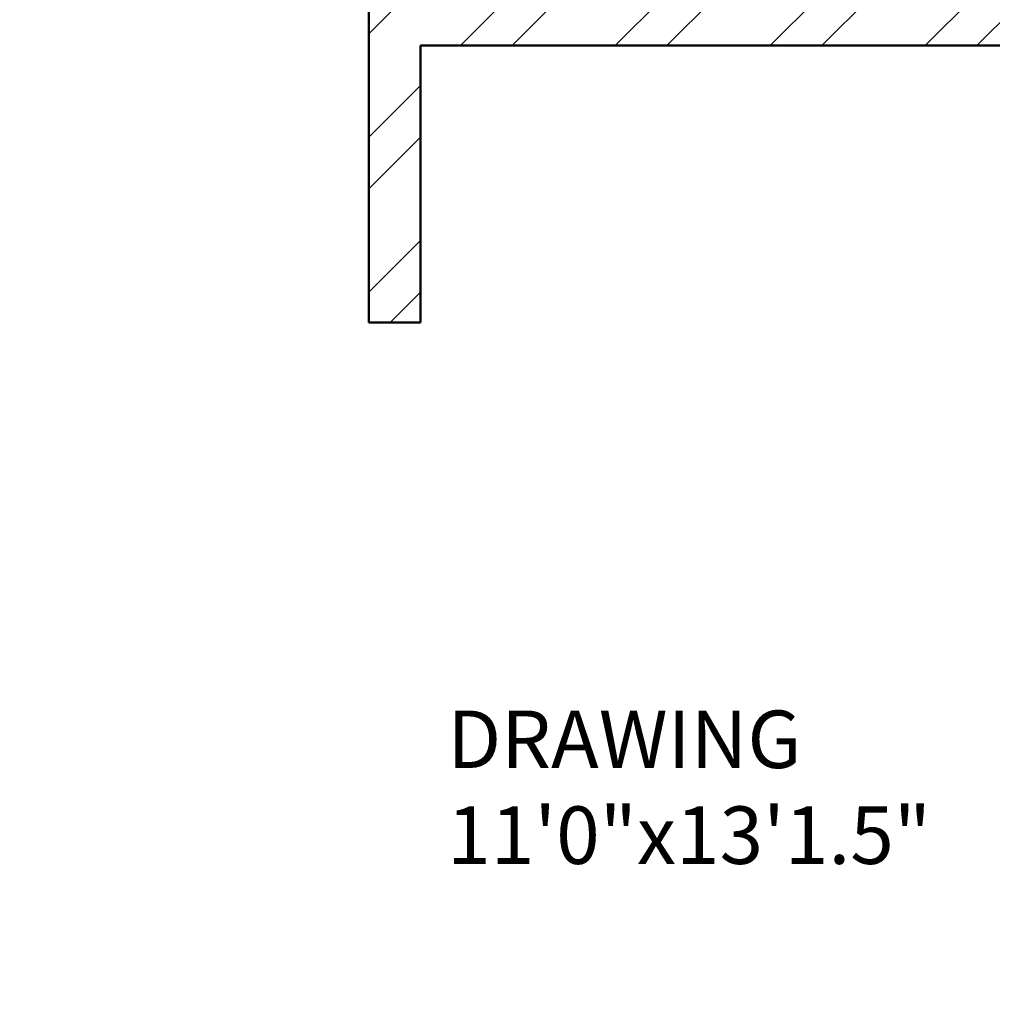
# Model space of a CAD drawing. Units: inches. Extents: x 963 to 2075, y 289 to 2657.
# Tile 73 of 98: x 1342 to 1426, y 2239 to 2325. Entities that reach past the tile are written whole.
import ezdxf

# ---------------------------------------------------------------- set-up
doc = ezdxf.new("R2010")
doc.units = ezdxf.units.IN
for name, color, linetype, lineweight in [('A-AREA-IDEN', 7, 'Continuous', 18), ('A-WALL', 7, 'Continuous', 50), ('A-WALL-PATT', 8, 'Continuous', 13)]:
    doc.layers.add(name, color=color, linetype=linetype, lineweight=lineweight)
doc.styles.get("Standard").update_dxf_attribs({"font": 'arial.ttf'})

msp = doc.modelspace()

# ---------------------------------------------------------------- hatches: boundary and pattern name
at = {"layer": 'A-WALL-PATT'}
h = msp.add_hatch(dxfattribs=at)
h.set_pattern_fill('ANSI32', color=256)
h.paths.add_polyline_path([(1296.922, 2558.318), (1203.922, 2558.318), (1203.922, 2493.818), (1191.533, 2493.818), (1191.533, 2489.318), (1211.063, 2489.318), (1211.063, 2492.02), (1211.063, 2493.818), (1208.422, 2493.818), (1208.422, 2553.818), (1292.422, 2553.818), (1292.422, 2538.863), (1296.922, 2538.863)])
h.paths.add_polyline_path([(1442.422, 2558.318), (1349.422, 2558.318), (1349.422, 2538.943), (1353.922, 2538.943), (1353.922, 2553.818), (1437.922, 2553.818), (1437.922, 2493.818), (1434.542, 2493.818), (1434.542, 2489.318), (1448.311, 2489.318), (1448.311, 2491.568), (1448.311, 2493.818), (1442.422, 2493.818)])
h.paths.add_polyline_path([(1415.554, 2491.568), (1415.554, 2493.818), (1340.941, 2493.818), (1340.941, 2489.318), (1371.922, 2489.318), (1371.922, 2378.318), (1367.596, 2378.318), (1367.596, 2373.818), (1371.922, 2373.818), (1371.922, 2355.185), (1376.422, 2355.185), (1376.422, 2489.318), (1415.554, 2489.318)])
h.paths.add_polyline_path([(1304.941, 2491.568), (1304.941, 2493.818), (1296.922, 2493.818), (1296.922, 2514.863), (1292.422, 2514.863), (1292.422, 2493.818), (1232.808, 2493.818), (1232.808, 2489.318), (1256.422, 2489.318), (1256.422, 2327.318), (1253.714, 2327.318), (1253.714, 2322.818), (1328.422, 2322.818), (1328.422, 2331.147), (1323.922, 2331.147), (1323.922, 2327.318), (1260.922, 2327.318), (1260.922, 2373.818), (1323.922, 2373.818), (1323.922, 2357.812), (1328.422, 2357.812), (1328.422, 2373.818), (1346.007, 2373.818), (1346.007, 2376.068), (1346.007, 2378.318), (1260.922, 2378.318), (1260.922, 2489.318), (1304.941, 2489.318)])
h.paths.add_polyline_path([(1226.654, 2327.318), (1124.422, 2327.318), (1124.422, 2347.447), (1119.922, 2347.447), (1119.922, 2322.818), (1163.422, 2322.818), (1163.422, 2305.435), (1165.672, 2305.435), (1167.922, 2305.435), (1167.922, 2322.818), (1226.654, 2322.818), (1226.654, 2325.068)])
h.paths.add_polyline_path([(1095.922, 2489.318), (1124.422, 2489.318), (1131.533, 2489.318), (1131.533, 2491.568), (1131.533, 2493.818), (1119.922, 2493.818), (1091.422, 2493.818), (1091.422, 2417.318), (1095.922, 2417.318), (1119.922, 2417.318), (1119.922, 2407.447), (1124.422, 2407.447), (1124.422, 2421.818), (1095.922, 2421.818)])
h.paths.add_polyline_path([(1512.922, 2558.318), (1508.422, 2558.318), (1508.422, 2493.818), (1503.401, 2493.818), (1503.401, 2489.318), (1508.422, 2489.318), (1508.422, 2327.318), (1376.422, 2327.318), (1376.422, 2330.273), (1371.922, 2330.273), (1371.922, 2298.744), (1376.422, 2298.744), (1376.422, 2322.818), (1508.422, 2322.818), (1508.422, 2165.318), (1504.255, 2165.318), (1504.255, 2160.818), (1508.422, 2160.818), (1508.422, 2108.318), (1512.922, 2108.318), (1512.922, 2160.818), (1516.182, 2160.818), (1516.182, 2163.068), (1516.182, 2165.318), (1512.922, 2165.318), (1512.922, 2322.818), (1644.922, 2322.818), (1644.922, 2298.744), (1649.422, 2298.744), (1649.422, 2322.818), (1649.422, 2330.944), (1647.172, 2330.944), (1644.922, 2330.944), (1644.922, 2327.318), (1512.922, 2327.318), (1512.922, 2489.318), (1516.759, 2489.318), (1516.759, 2491.568), (1516.759, 2493.818), (1512.922, 2493.818)])
h.paths.add_polyline_path([(1671.922, 2558.318), (1578.922, 2558.318), (1578.922, 2493.818), (1573.526, 2493.818), (1573.526, 2489.318), (1586.537, 2489.318), (1586.537, 2491.568), (1586.537, 2493.818), (1583.422, 2493.818), (1583.422, 2553.818), (1667.422, 2553.818), (1667.422, 2541.109), (1671.922, 2541.109)])
h.paths.add_polyline_path([(1681.257, 2493.818), (1671.922, 2493.818), (1671.922, 2517.109), (1667.422, 2517.109), (1667.422, 2493.818), (1610.218, 2493.818), (1610.218, 2489.318), (1644.922, 2489.318), (1644.922, 2357.865), (1649.422, 2357.865), (1649.422, 2373.818), (1652.203, 2373.818), (1652.203, 2375.827), (1652.203, 2378.318), (1649.422, 2378.318), (1649.422, 2489.318), (1681.257, 2489.318), (1681.257, 2491.568)])
h.paths.add_polyline_path([(1821.922, 2558.318), (1728.922, 2558.318), (1728.922, 2541), (1733.422, 2541), (1733.422, 2553.818), (1817.422, 2553.818), (1817.422, 2493.818), (1813.507, 2493.818), (1813.507, 2489.318), (1830.078, 2489.318), (1830.078, 2491.568), (1830.078, 2493.818), (1821.922, 2493.818)])
h.paths.add_polyline_path([(1794.244, 2493.818), (1717.257, 2493.818), (1717.257, 2489.318), (1760.422, 2489.318), (1760.422, 2378.318), (1674.401, 2378.318), (1674.401, 2373.818), (1692.922, 2373.818), (1692.922, 2356.954), (1697.422, 2356.954), (1697.422, 2373.818), (1760.422, 2373.818), (1760.422, 2327.318), (1697.422, 2327.318), (1697.422, 2333.341), (1692.922, 2333.341), (1692.922, 2322.818), (1768.037, 2322.818), (1768.037, 2325.068), (1768.037, 2327.318), (1764.922, 2327.318), (1764.922, 2489.318), (1794.244, 2489.318)])
h.paths.add_polyline_path([(1733.422, 2517), (1728.922, 2517), (1728.922, 2493.818), (1733.422, 2493.818)], flags=17)
h.paths.add_polyline_path([(1929.922, 2493.818), (1890.078, 2493.818), (1890.078, 2489.318), (1896.922, 2489.318), (1925.422, 2489.318), (1925.422, 2421.818), (1896.922, 2421.818), (1896.922, 2408.318), (1901.422, 2408.318), (1901.422, 2417.318), (1925.422, 2417.318), (1929.922, 2417.318)])
h.paths.add_polyline_path([(1901.422, 2348.318), (1896.922, 2348.318), (1896.922, 2327.318), (1800.423, 2327.318), (1800.423, 2322.818), (1853.422, 2322.818), (1853.422, 2309.453), (1857.922, 2309.453), (1857.922, 2322.818), (1901.422, 2322.818)])
h.paths.add_polyline_path([(1857.922, 2249.453), (1853.422, 2249.453), (1853.422, 2214.818), (1686.309, 2214.818), (1686.309, 2210.318), (1853.422, 2210.318), (1853.422, 2202.134), (1857.922, 2202.134), (1857.922, 2210.318)])
h.paths.add_polyline_path([(1857.922, 2142.134), (1853.422, 2142.134), (1853.422, 2115.422), (1841.422, 2115.422), (1841.422, 2088.531), (1841.422, 2046.949), (1845.922, 2046.949), (1845.922, 2110.922), (1905.922, 2110.922), (1905.922, 2092.517), (1910.422, 2092.517), (1910.422, 2115.422), (1857.922, 2115.422)])
h.paths.add_polyline_path([(1532.436, 1482.342), (1573.456, 1482.342), (1573.456, 1501), (1532.436, 1501)], flags=9)
h.paths.add_polyline_path([(1438.658, 1486.302), (1479.678, 1486.302), (1479.678, 1504.96), (1438.658, 1504.96)], flags=9)
h.paths.add_polyline_path([(1411.215, 1365.308), (1659.139, 1365.308), (1659.139, 1402.401), (1411.215, 1402.401)], flags=9)
h.paths.add_polyline_path([(1185.671, 2296.298), (1248.16, 2296.298), (1248.16, 2314.955), (1185.671, 2314.955)], flags=9)
h.paths.add_polyline_path([(1177.31, 2187.35), (1216.15, 2187.35), (1216.15, 2206.007), (1177.31, 2206.007)], flags=9)
h.paths.add_polyline_path([(1295.101, 1602.083), (1328.26, 1602.083), (1328.26, 1620.741), (1295.101, 1620.741)], flags=9)
h.paths.add_polyline_path([(1525.126, 2005.99), (1558.39, 2005.99), (1558.39, 2024.648), (1525.126, 2024.648)], flags=9)
h.paths.add_polyline_path([(1459.606, 1977.125), (1472.195, 1977.125), (1472.195, 1987.429), (1459.606, 1987.429)], flags=9)
h.paths.add_polyline_path([(1467.815, 2053.676), (1480.018, 2053.676), (1480.018, 2063.979), (1467.815, 2063.979)], flags=9)
h.paths.add_polyline_path([(1555.184, 2119.02), (1584.563, 2119.02), (1584.563, 2137.678), (1555.184, 2137.678)], flags=25)
h.paths.add_polyline_path([(1405.389, 2115.291), (1444.478, 2115.291), (1444.478, 2133.948), (1405.389, 2133.948)], flags=25)
h.paths.add_polyline_path([(1698.482, 2004.259), (1727.695, 2004.259), (1727.695, 2022.916), (1698.482, 2022.916)], flags=9)
h.paths.add_polyline_path([(1612.158, 1972.855), (1629.016, 1972.855), (1629.016, 1983.159), (1612.158, 1983.159)], flags=9)
h.paths.add_polyline_path([(1608.289, 2060.036), (1625.147, 2060.036), (1625.147, 2070.34), (1608.289, 2070.34)], flags=9)
h.paths.add_polyline_path([(1527.954, 1684.402), (1566.795, 1684.402), (1566.795, 1703.06), (1527.954, 1703.06)], flags=9)
h.paths.add_polyline_path([(1422.792, 1683.59), (1461.633, 1683.59), (1461.633, 1702.247), (1422.792, 1702.247)], flags=9)
h.paths.add_polyline_path([(1531.262, 1732.459), (1574.015, 1732.459), (1574.015, 1751.116), (1531.262, 1751.116)], flags=9)
h.paths.add_polyline_path([(1402.872, 1732.845), (1439.799, 1732.845), (1439.799, 1751.502), (1402.872, 1751.502)], flags=9)
h.paths.add_polyline_path([(1243.122, 1923.132), (1281.962, 1923.132), (1281.962, 1941.79), (1243.122, 1941.79)], flags=9)
h.paths.add_polyline_path([(1181.752, 1792.268), (1244.241, 1792.268), (1244.241, 1810.926), (1181.752, 1810.926)], flags=9)
h.paths.add_polyline_path([(1265.822, 1670.3), (1316.071, 1670.3), (1316.071, 1688.957), (1265.822, 1688.957)], flags=9)
h.paths.add_polyline_path([(1140.263, 1676.054), (1179.104, 1676.054), (1179.104, 1694.711), (1140.263, 1694.711)], flags=9)
h.paths.add_polyline_path([(1107.49, 1490.889), (1143.374, 1490.889), (1143.374, 1509.546), (1107.49, 1509.546)], flags=9)
h.paths.add_polyline_path([(1217.584, 1483.899), (1246.741, 1483.899), (1246.741, 1502.556), (1217.584, 1502.556)], flags=9)
h.paths.add_polyline_path([(1389.21, 1486.919), (1418.367, 1486.919), (1418.367, 1505.576), (1389.21, 1505.576)], flags=9)
h.paths.add_polyline_path([(1672.208, 1602.083), (1705.366, 1602.083), (1705.366, 1620.741), (1672.208, 1620.741)], flags=9)
h.paths.add_polyline_path([(1752.082, 1522.638), (1781.24, 1522.638), (1781.24, 1541.295), (1752.082, 1541.295)], flags=9)
h.paths.add_polyline_path([(1848.275, 1491.26), (1884.158, 1491.26), (1884.158, 1509.918), (1848.275, 1509.918)], flags=9)
h.paths.add_polyline_path([(1822.47, 1685.62), (1861.31, 1685.62), (1861.31, 1704.278), (1822.47, 1704.278)], flags=9)
h.paths.add_polyline_path([(1713.195, 1672.232), (1763.444, 1672.232), (1763.444, 1690.889), (1713.195, 1690.889)], flags=9)
h.paths.add_polyline_path([(1736.619, 1790.578), (1799.109, 1790.578), (1799.109, 1809.235), (1736.619, 1809.235)], flags=9)
h.paths.add_polyline_path([(1691.491, 1916.355), (1730.332, 1916.355), (1730.332, 1935.013), (1691.491, 1935.013)], flags=9)
h.paths.add_polyline_path([(1764.872, 1973.922), (1794.306, 1973.922), (1794.306, 1992.58), (1764.872, 1992.58)], flags=9)
h.paths.add_polyline_path([(1767.854, 2034.017), (1797.288, 2034.017), (1797.288, 2052.674), (1767.854, 2052.674)], flags=9)
h.paths.add_polyline_path([(1851.593, 2060.331), (1880.751, 2060.331), (1880.751, 2078.989), (1851.593, 2078.989)], flags=25)
h.paths.add_polyline_path([(1688.491, 2086.874), (1727.332, 2086.874), (1727.332, 2105.531), (1688.491, 2105.531)], flags=9)
h.paths.add_polyline_path([(1537.743, 2293.581), (1580.495, 2293.581), (1580.495, 2312.239), (1537.743, 2312.239)], flags=25)
h.paths.add_polyline_path([(1425.587, 2296.109), (1468.34, 2296.109), (1468.34, 2314.766), (1425.587, 2314.766)], flags=25)
h.paths.add_polyline_path([(1278.518, 2004.184), (1307.72, 2004.184), (1307.72, 2022.841), (1278.518, 2022.841)], flags=9)
h.paths.add_polyline_path([(1193.282, 1973.635), (1222.715, 1973.635), (1222.715, 1992.292), (1193.282, 1992.292)], flags=9)
h.paths.add_polyline_path([(1192.411, 2040.577), (1221.845, 2040.577), (1221.845, 2059.234), (1192.411, 2059.234)], flags=9)
h.paths.add_polyline_path([(1130.603, 1951.393), (1159.76, 1951.393), (1159.76, 1970.05), (1130.603, 1970.05)], flags=9)
h.paths.add_polyline_path([(1132.827, 2052.494), (1161.984, 2052.494), (1161.984, 2071.151), (1132.827, 2071.151)], flags=9)
h.paths.add_polyline_path([(1265.128, 2334.619), (1315.377, 2334.619), (1315.377, 2353.277), (1265.128, 2353.277)], flags=25)
h.paths.add_polyline_path([(1136.741, 2330.785), (1175.582, 2330.785), (1175.582, 2349.443), (1136.741, 2349.443)], flags=9)
h.paths.add_polyline_path([(1287.422, 2417.204), (1320.58, 2417.204), (1320.58, 2435.861), (1287.422, 2435.861)], flags=25)
h.paths.add_polyline_path([(1430.988, 2329.159), (1469.828, 2329.159), (1469.828, 2347.816), (1430.988, 2347.816)], flags=25)
h.paths.add_polyline_path([(1525.424, 2329.213), (1564.264, 2329.213), (1564.264, 2347.87), (1525.424, 2347.87)], flags=25)
h.paths.add_polyline_path([(1684.525, 2382.799), (1717.683, 2382.799), (1717.683, 2401.457), (1684.525, 2401.457)], flags=25)
h.paths.add_polyline_path([(1704.805, 2340.293), (1755.054, 2340.293), (1755.054, 2358.95), (1704.805, 2358.95)], flags=25)
h.paths.add_polyline_path([(1694.113, 2287.757), (1756.602, 2287.757), (1756.602, 2306.414), (1694.113, 2306.414)], flags=9)
h.paths.add_polyline_path([(1815.778, 2329.861), (1854.618, 2329.861), (1854.618, 2348.518), (1815.778, 2348.518)], flags=9)
h.paths.add_polyline_path([(1842.873, 2514.256), (1878.756, 2514.256), (1878.756, 2532.914), (1842.873, 2532.914)], flags=9)
h.paths.add_polyline_path([(1769.513, 2531.447), (1798.671, 2531.447), (1798.671, 2550.104), (1769.513, 2550.104)], flags=25)
h.paths.add_polyline_path([(1594.772, 2518.468), (1623.93, 2518.468), (1623.93, 2537.125), (1594.772, 2537.125)], flags=25)
h.paths.add_polyline_path([(1520.723, 2516.185), (1556.606, 2516.185), (1556.606, 2534.842), (1520.723, 2534.842)], flags=25)
h.paths.add_polyline_path([(1464.456, 2516.694), (1500.34, 2516.694), (1500.34, 2535.351), (1464.456, 2535.351)], flags=25)
h.paths.add_polyline_path([(1365.696, 2528.97), (1394.854, 2528.97), (1394.854, 2547.627), (1365.696, 2547.627)], flags=25)
h.paths.add_polyline_path([(1222.838, 2516.231), (1251.995, 2516.231), (1251.995, 2534.889), (1222.838, 2534.889)], flags=25)
h.paths.add_polyline_path([(1104.545, 2509.6), (1140.429, 2509.6), (1140.429, 2528.257), (1104.545, 2528.257)], flags=9)
h = msp.add_hatch(dxfattribs=at)
h.set_pattern_fill('ANSI32', color=256)
h.paths.add_polyline_path([(1335.968, 2212.568), (1335.968, 2214.818), (1167.922, 2214.818), (1167.922, 2245.435), (1163.422, 2245.435), (1163.422, 2210.318), (1163.422, 2194.812), (1167.922, 2194.812), (1167.922, 2210.318), (1335.968, 2210.318)])
h.paths.add_polyline_path([(1532.436, 1482.342), (1573.456, 1482.342), (1573.456, 1501), (1532.436, 1501)], flags=9)
h.paths.add_polyline_path([(1438.658, 1486.302), (1479.678, 1486.302), (1479.678, 1504.96), (1438.658, 1504.96)], flags=9)
h.paths.add_polyline_path([(1411.215, 1365.308), (1659.139, 1365.308), (1659.139, 1402.401), (1411.215, 1402.401)], flags=9)
h.paths.add_polyline_path([(1185.671, 2296.298), (1248.16, 2296.298), (1248.16, 2314.955), (1185.671, 2314.955)], flags=9)
h.paths.add_polyline_path([(1177.31, 2187.35), (1216.15, 2187.35), (1216.15, 2206.007), (1177.31, 2206.007)], flags=9)
h.paths.add_polyline_path([(1295.101, 1602.083), (1328.26, 1602.083), (1328.26, 1620.741), (1295.101, 1620.741)], flags=9)
h.paths.add_polyline_path([(1525.126, 2005.99), (1558.39, 2005.99), (1558.39, 2024.648), (1525.126, 2024.648)], flags=9)
h.paths.add_polyline_path([(1459.606, 1977.125), (1472.195, 1977.125), (1472.195, 1987.429), (1459.606, 1987.429)], flags=9)
h.paths.add_polyline_path([(1467.815, 2053.676), (1480.018, 2053.676), (1480.018, 2063.979), (1467.815, 2063.979)], flags=9)
h.paths.add_polyline_path([(1555.184, 2119.02), (1584.563, 2119.02), (1584.563, 2137.678), (1555.184, 2137.678)], flags=9)
h.paths.add_polyline_path([(1405.389, 2115.291), (1444.478, 2115.291), (1444.478, 2133.948), (1405.389, 2133.948)], flags=9)
h.paths.add_polyline_path([(1698.482, 2004.259), (1727.695, 2004.259), (1727.695, 2022.916), (1698.482, 2022.916)], flags=9)
h.paths.add_polyline_path([(1612.158, 1972.855), (1629.016, 1972.855), (1629.016, 1983.159), (1612.158, 1983.159)], flags=9)
h.paths.add_polyline_path([(1608.289, 2060.036), (1625.147, 2060.036), (1625.147, 2070.34), (1608.289, 2070.34)], flags=9)
h.paths.add_polyline_path([(1527.954, 1684.402), (1566.795, 1684.402), (1566.795, 1703.06), (1527.954, 1703.06)], flags=9)
h.paths.add_polyline_path([(1422.792, 1683.59), (1461.633, 1683.59), (1461.633, 1702.247), (1422.792, 1702.247)], flags=9)
h.paths.add_polyline_path([(1531.262, 1732.459), (1574.015, 1732.459), (1574.015, 1751.116), (1531.262, 1751.116)], flags=9)
h.paths.add_polyline_path([(1402.872, 1732.845), (1439.799, 1732.845), (1439.799, 1751.502), (1402.872, 1751.502)], flags=9)
h.paths.add_polyline_path([(1243.122, 1923.132), (1281.962, 1923.132), (1281.962, 1941.79), (1243.122, 1941.79)], flags=9)
h.paths.add_polyline_path([(1181.752, 1792.268), (1244.241, 1792.268), (1244.241, 1810.926), (1181.752, 1810.926)], flags=9)
h.paths.add_polyline_path([(1265.822, 1670.3), (1316.071, 1670.3), (1316.071, 1688.957), (1265.822, 1688.957)], flags=9)
h.paths.add_polyline_path([(1140.263, 1676.054), (1179.104, 1676.054), (1179.104, 1694.711), (1140.263, 1694.711)], flags=9)
h.paths.add_polyline_path([(1107.49, 1490.889), (1143.374, 1490.889), (1143.374, 1509.546), (1107.49, 1509.546)], flags=9)
h.paths.add_polyline_path([(1217.584, 1483.899), (1246.741, 1483.899), (1246.741, 1502.556), (1217.584, 1502.556)], flags=9)
h.paths.add_polyline_path([(1389.21, 1486.919), (1418.367, 1486.919), (1418.367, 1505.576), (1389.21, 1505.576)], flags=9)
h.paths.add_polyline_path([(1672.208, 1602.083), (1705.366, 1602.083), (1705.366, 1620.741), (1672.208, 1620.741)], flags=9)
h.paths.add_polyline_path([(1752.082, 1522.638), (1781.24, 1522.638), (1781.24, 1541.295), (1752.082, 1541.295)], flags=9)
h.paths.add_polyline_path([(1848.275, 1491.26), (1884.158, 1491.26), (1884.158, 1509.918), (1848.275, 1509.918)], flags=9)
h.paths.add_polyline_path([(1822.47, 1685.62), (1861.31, 1685.62), (1861.31, 1704.278), (1822.47, 1704.278)], flags=9)
h.paths.add_polyline_path([(1713.195, 1672.232), (1763.444, 1672.232), (1763.444, 1690.889), (1713.195, 1690.889)], flags=9)
h.paths.add_polyline_path([(1736.619, 1790.578), (1799.109, 1790.578), (1799.109, 1809.235), (1736.619, 1809.235)], flags=9)
h.paths.add_polyline_path([(1691.491, 1916.355), (1730.332, 1916.355), (1730.332, 1935.013), (1691.491, 1935.013)], flags=9)
h.paths.add_polyline_path([(1764.872, 1973.922), (1794.306, 1973.922), (1794.306, 1992.58), (1764.872, 1992.58)], flags=9)
h.paths.add_polyline_path([(1767.854, 2034.017), (1797.288, 2034.017), (1797.288, 2052.674), (1767.854, 2052.674)], flags=9)
h.paths.add_polyline_path([(1851.593, 2060.331), (1880.751, 2060.331), (1880.751, 2078.989), (1851.593, 2078.989)], flags=9)
h.paths.add_polyline_path([(1688.491, 2086.874), (1727.332, 2086.874), (1727.332, 2105.531), (1688.491, 2105.531)], flags=9)
h.paths.add_polyline_path([(1537.743, 2293.581), (1580.495, 2293.581), (1580.495, 2312.239), (1537.743, 2312.239)], flags=9)
h.paths.add_polyline_path([(1425.587, 2296.109), (1468.34, 2296.109), (1468.34, 2314.766), (1425.587, 2314.766)], flags=9)
h.paths.add_polyline_path([(1278.518, 2004.184), (1307.72, 2004.184), (1307.72, 2022.841), (1278.518, 2022.841)], flags=9)
h.paths.add_polyline_path([(1193.282, 1973.635), (1222.715, 1973.635), (1222.715, 1992.292), (1193.282, 1992.292)], flags=9)
h.paths.add_polyline_path([(1192.411, 2040.577), (1221.845, 2040.577), (1221.845, 2059.234), (1192.411, 2059.234)], flags=9)
h.paths.add_polyline_path([(1130.603, 1951.393), (1159.76, 1951.393), (1159.76, 1970.05), (1130.603, 1970.05)], flags=9)
h.paths.add_polyline_path([(1132.827, 2052.494), (1161.984, 2052.494), (1161.984, 2071.151), (1132.827, 2071.151)], flags=9)
h.paths.add_polyline_path([(1265.128, 2334.619), (1315.377, 2334.619), (1315.377, 2353.277), (1265.128, 2353.277)], flags=9)
h.paths.add_polyline_path([(1136.741, 2330.785), (1175.582, 2330.785), (1175.582, 2349.443), (1136.741, 2349.443)], flags=9)
h.paths.add_polyline_path([(1287.422, 2417.204), (1320.58, 2417.204), (1320.58, 2435.861), (1287.422, 2435.861)], flags=9)
h.paths.add_polyline_path([(1430.988, 2329.159), (1469.828, 2329.159), (1469.828, 2347.816), (1430.988, 2347.816)], flags=9)
h.paths.add_polyline_path([(1525.424, 2329.213), (1564.264, 2329.213), (1564.264, 2347.87), (1525.424, 2347.87)], flags=9)
h.paths.add_polyline_path([(1684.525, 2382.799), (1717.683, 2382.799), (1717.683, 2401.457), (1684.525, 2401.457)], flags=9)
h.paths.add_polyline_path([(1704.805, 2340.293), (1755.054, 2340.293), (1755.054, 2358.95), (1704.805, 2358.95)], flags=9)
h.paths.add_polyline_path([(1694.113, 2287.757), (1756.602, 2287.757), (1756.602, 2306.414), (1694.113, 2306.414)], flags=9)
h.paths.add_polyline_path([(1815.778, 2329.861), (1854.618, 2329.861), (1854.618, 2348.518), (1815.778, 2348.518)], flags=9)
h.paths.add_polyline_path([(1842.873, 2514.256), (1878.756, 2514.256), (1878.756, 2532.914), (1842.873, 2532.914)], flags=9)
h.paths.add_polyline_path([(1769.513, 2531.447), (1798.671, 2531.447), (1798.671, 2550.104), (1769.513, 2550.104)], flags=9)
h.paths.add_polyline_path([(1594.772, 2518.468), (1623.93, 2518.468), (1623.93, 2537.125), (1594.772, 2537.125)], flags=9)
h.paths.add_polyline_path([(1520.723, 2516.185), (1556.606, 2516.185), (1556.606, 2534.842), (1520.723, 2534.842)], flags=9)
h.paths.add_polyline_path([(1464.456, 2516.694), (1500.34, 2516.694), (1500.34, 2535.351), (1464.456, 2535.351)], flags=9)
h.paths.add_polyline_path([(1365.696, 2528.97), (1394.854, 2528.97), (1394.854, 2547.627), (1365.696, 2547.627)], flags=9)
h.paths.add_polyline_path([(1222.838, 2516.231), (1251.995, 2516.231), (1251.995, 2534.889), (1222.838, 2534.889)], flags=9)
h.paths.add_polyline_path([(1104.545, 2509.6), (1140.429, 2509.6), (1140.429, 2528.257), (1104.545, 2528.257)], flags=9)

# ---------------------------------------------------------------- linework, layer by layer
at = {"layer": 'A-WALL'}
for p, q in [((1371.922, 2330.273), (1371.922, 2298.744)), ((1376.422, 2322.818), (1508.422, 2322.818)), ((1376.422, 2322.818), (1376.422, 2298.744)), ((1371.922, 2298.744), (1376.422, 2298.744))]:
    msp.add_line(p, q, dxfattribs=at)

# ---------------------------------------------------------------- texts
at = {"layer": 'A-AREA-IDEN', "insert": (1378.751, 2265.014), "char_height": 5, "attachment_point": 1}
msp.add_mtext_dynamic_manual_height_columns('DRAWING\\P11\'0"x13\'1.5"', width=175.54917, gutter_width=12.5, heights=[0], dxfattribs=at)

doc.saveas('drawing.dxf')
